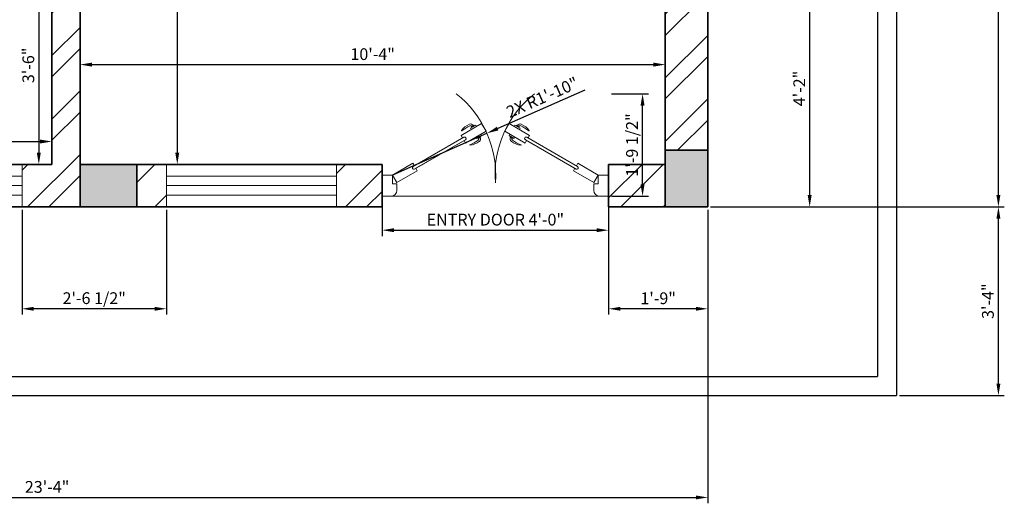
# Model space of a CAD drawing. Units: inches. Extents: x -138 to 270, y 8284 to 8764.
# Tile 5 of 10: x 61 to 270, y 8284 to 8387. Entities that reach past the tile are written whole.
import ezdxf

# ---------------------------------------------------------------- set-up
doc = ezdxf.new("R2010")
doc.units = ezdxf.units.IN
for name, color, linetype, lineweight in [('A-ANNO-DIMS', 2, 'Continuous', 18), ('C-PROP', 7, 'Continuous', 25), ('DOOR', 32, 'Continuous', 15), ('WALL', 8, 'Continuous', 35), ('WINDOW', 151, 'Continuous', 15)]:
    doc.layers.add(name, color=color, linetype=linetype, lineweight=lineweight)
doc.layers.add('A-COLS', color=252, linetype='Continuous', lineweight=35, true_color=0x939598)
doc.layers.add('A-WALL-PATT', color=32, linetype='Continuous', lineweight=9, true_color=0xbc761a)
doc.styles.get("Standard").update_dxf_attribs({"font": 'arial.ttf'})
doc.dimstyles.new('ISO-25', dxfattribs={"dimtxt": 2.5, "dimasz": 2.5, "dimexe": 1.25, "dimexo": 0.625, "dimtad": 1, "dimdec": 0, "dimlunit": 3, "dimtxsty": 'Standard', "dimcen": 2.5, "dimadec": 0, "dimazin": 0, "dimtfac": 1, "dimtdec": 0, "dimtmove": 0, "dimatfit": 3, "dimfxl": 1, "dimarcsym": 0})

# ---------------------------------------------------------------- blocks, each defined once
blk = doc.blocks.new('A$C441550E7')
at = {"layer": 'DOOR'}
for p, q in [((16.75, 12.91), (21.08, 15.41)), ((18.76, 14.43), (19.84, 15.05)), ((18.93, 14.75), (19.47, 15.06)), ((18.93, 14.75), (19.03, 14.58)), ((18.93, 14.75), (18.93, 14.75)), ((19.2, 14.9), (19.2, 14.9)), ((19.47, 15.06), (19.57, 14.9)), ((19.84, 15.05), (20, 14.78)), ((22.02, 13.78), (21.08, 15.41)), ((25.98, 13.78), (26.92, 15.41)), ((31.25, 12.91), (26.92, 15.41)), ((28.16, 15.05), (28, 14.78)), ((29.24, 14.43), (28.16, 15.05)), ((28.53, 15.06), (28.43, 14.9)), ((29.07, 14.75), (28.53, 15.06)), ((28.8, 14.9), (28.8, 14.9)), ((29.07, 14.75), (28.97, 14.58)), ((29.07, 14.75), (29.07, 14.75)), ((6.56, 6.3), (17.33, 12.52)), ((17.06, 12.36), (16.75, 12.91)), ((17.69, 11.28), (22.02, 13.78)), ((18.76, 14.43), (18.91, 14.16)), ((20.01, 12.26), (19.85, 12.53)), ((20.01, 12.26), (21.09, 12.89)), ((20.37, 12.26), (20.91, 12.57)), ((20.91, 12.57), (20.82, 12.73)), ((21.09, 12.89), (20.93, 13.16)), ((30.31, 11.28), (25.98, 13.78)), ((26.91, 12.89), (27.07, 13.16)), ((27.99, 12.26), (26.91, 12.89)), ((27.09, 12.57), (27.18, 12.73)), ((27.63, 12.26), (27.09, 12.57)), ((27.99, 12.26), (28.15, 12.53)), ((29.24, 14.43), (29.09, 14.16)), ((41.44, 6.3), (30.67, 12.52)), ((30.94, 12.36), (31.25, 12.91)), ((17.64, 11.98), (6.87, 5.76)), ((7.14, 5.92), (17.37, 11.82)), ((17.69, 11.28), (17.37, 11.82)), ((17.76, 12.41), (17.76, 12.41)), ((20.37, 12.26), (20.28, 12.42)), ((20.37, 12.26), (20.37, 12.26)), ((20.64, 12.41), (20.64, 12.41)), ((27.36, 12.41), (27.36, 12.41)), ((27.63, 12.26), (27.72, 12.42)), ((27.63, 12.26), (27.63, 12.26)), ((30.24, 12.41), (30.24, 12.41)), ((30.31, 11.28), (30.63, 11.82)), ((30.36, 11.98), (41.13, 5.76)), ((40.86, 5.92), (30.63, 11.82)), ((6.52, 7), (2.19, 4.5)), ((6.83, 6.46), (6.52, 7)), ((41.17, 6.46), (41.48, 7)), ((41.48, 7), (45.81, 4.5)), ((0, 0), (0, 4.5)), ((0, 4.5), (2.19, 4.5)), ((2.19, 2.62), (2.19, 4.5)), ((3.12, 2.88), (2.19, 4.5)), ((7.46, 5.38), (3.12, 2.88)), ((6.45, 5.88), (6.45, 5.88)), ((7.46, 5.38), (7.14, 5.92)), ((40.54, 5.38), (40.86, 5.92)), ((40.54, 5.38), (44.87, 2.88)), ((41.55, 5.88), (41.55, 5.88)), ((44.87, 2.88), (45.81, 4.5)), ((48, 4.5), (45.81, 4.5)), ((45.81, 2.62), (45.81, 4.5)), ((48, 0), (48, 4.5)), ((2.19, 2.62), (3.12, 2.62)), ((3.12, 1.25), (3.12, 2.62)), ((44.87, 1.25), (44.87, 2.62)), ((45.81, 2.62), (44.87, 2.62)), ((0, 0), (1.87, 0)), ((0, 0), (48, 0)), ((48, 0), (46.12, 0))]:
    blk.add_line(p, q, dxfattribs=at)
at = {"layer": 'DOOR', "ltscale": 0.1}
for centre, start, end in [((2.3, 4.56), 355.5279, 52.0858), ((45.7, 4.56), 127.9142, 184.4721)]:
    blk.add_arc(centre, 21.77, start, end, dxfattribs=at)
at = {"layer": 'DOOR'}
for centre, radius, start, end in [((19.83, 11.88), 3.63, 111.4546, 145.7774), ((22.15, 7.07), 8.61, 114.2033, 127.709), ((18.77, 14.74), 0.592, 22.7059, 117.5689), ((18.78, 14.66), 0.312, 30, 120), ((29.23, 14.74), 0.592, 62.4311, 157.2941), ((29.22, 14.66), 0.312, 60, 150), ((25.85, 7.07), 8.61, 52.291, 65.7967), ((28.17, 11.88), 3.63, 34.2226, 68.5454), ((16.85, 13.9), 0.0372, 138.2373, 332.5518), ((17.49, 12.25), 0.312, 30, 120), ((30.51, 12.25), 0.312, 60, 150), ((31.15, 13.9), 0.0372, 207.4482, 41.7627), ((17.49, 12.25), 0.312, 300, 30), ((18.6, 10.88), 0.0372, 87.4482, 281.7627), ((15.33, 18.88), 8.61, 292.291, 305.7967), ((18.34, 14.46), 3.63, 274.2226, 308.5454), ((20.22, 12.17), 0.312, 300, 30), ((20.29, 12.12), 0.592, 302.4311, 37.2941), ((27.71, 12.12), 0.592, 142.7059, 237.5689), ((29.66, 14.46), 3.63, 231.4546, 265.7774), ((27.78, 12.17), 0.312, 150, 240), ((32.67, 18.88), 8.61, 234.2033, 247.709), ((29.4, 10.88), 0.0372, 258.2373, 92.5518), ((30.51, 12.25), 0.312, 150, 240), ((6.72, 6.03), 0.312, 120, 210), ((41.28, 6.03), 0.312, 330, 60), ((6.72, 6.03), 0.312, 210, 300), ((41.28, 6.03), 0.312, 240, 330), ((1.87, 1.25), 1.25, 270, 0), ((46.12, 1.25), 1.25, 180, 270)]:
    blk.add_arc(centre, radius, start, end, dxfattribs=at)
blk = doc.blocks.new('*D22')
at = {"layer": 'A-ANNO-DIMS', "color": 0, "lineweight": -2, "transparency": 16777216}
for p, q in [((94.04, 8484.24), (93.42, 8484.24)), ((94.67, 8481.74), (94.67, 8358.74)), ((94.04, 8356.24), (93.42, 8356.24))]:
    blk.add_line(p, q, dxfattribs=at)
at = {"layer": 'A-ANNO-DIMS', "color": 0, "transparency": 16777216}
for points in [[(94.25, 8481.74), (95.09, 8481.74), (94.67, 8484.24)], [(94.25, 8358.74), (95.09, 8358.74), (94.67, 8356.24)]]:
    blk.add_solid(points, dxfattribs=at)
at = {"layer": 'Defpoints', "color": 0, "transparency": 16777216}
for p in [(94.67, 8484.24), (94.67, 8356.24), (94.67, 8356.24)]:
    blk.add_point(p, dxfattribs=at)
at = {"layer": 'A-ANNO-DIMS', "color": 0, "transparency": 16777216, "insert": (92.77, 8420.24), "char_height": 2.5, "attachment_point": 5, "rotation": 90}
blk.add_mtext('10\'-8"', dxfattribs=at)
blk = doc.blocks.new('*D23')
at = {"layer": 'A-ANNO-DIMS', "color": 0, "lineweight": -2, "transparency": 16777216}
for p, q in [((74.08, 8376.44), (74.08, 8378.65)), ((198.08, 8376.44), (198.08, 8378.65)), ((76.58, 8377.4), (195.58, 8377.4))]:
    blk.add_line(p, q, dxfattribs=at)
at = {"layer": 'A-ANNO-DIMS', "color": 0, "transparency": 16777216}
for points in [[(76.58, 8377.82), (76.58, 8376.98), (74.08, 8377.4)], [(195.58, 8377.82), (195.58, 8376.98), (198.08, 8377.4)]]:
    blk.add_solid(points, dxfattribs=at)
at = {"layer": 'Defpoints', "color": 0, "transparency": 16777216}
for p in [(74.08, 8375.82), (198.08, 8377.4), (198.08, 8375.82)]:
    blk.add_point(p, dxfattribs=at)
at = {"layer": 'A-ANNO-DIMS', "color": 0, "transparency": 16777216, "insert": (136.08, 8379.3), "char_height": 2.5, "attachment_point": 5}
blk.add_mtext('10\'-4"', dxfattribs=at)
blk = doc.blocks.new('*D24')
at = {"layer": 'A-ANNO-DIMS', "color": 0, "lineweight": -2, "transparency": 16777216}
for p, q in [((32.08, 8356.87), (32.08, 8362.34)), ((68.08, 8356.87), (68.08, 8362.34)), ((34.58, 8361.09), (65.58, 8361.09))]:
    blk.add_line(p, q, dxfattribs=at)
at = {"layer": 'A-ANNO-DIMS', "color": 0, "transparency": 16777216}
for points in [[(34.58, 8361.51), (34.58, 8360.67), (32.08, 8361.09)], [(65.58, 8361.51), (65.58, 8360.67), (68.08, 8361.09)]]:
    blk.add_solid(points, dxfattribs=at)
at = {"layer": 'Defpoints', "color": 0, "transparency": 16777216}
for p in [(68.08, 8361.09), (32.08, 8356.24), (68.08, 8356.24)]:
    blk.add_point(p, dxfattribs=at)
at = {"layer": 'A-ANNO-DIMS', "color": 0, "transparency": 16777216, "insert": (50.08, 8362.99), "char_height": 2.5, "attachment_point": 5}
blk.add_mtext("3'", dxfattribs=at)
blk = doc.blocks.new('*D25')
at = {"layer": 'A-ANNO-DIMS', "color": 0, "lineweight": -2, "transparency": 16777216}
for p, q in [((67.45, 8398.24), (64.08, 8398.24)), ((65.33, 8395.74), (65.33, 8358.74)), ((67.45, 8356.24), (64.08, 8356.24))]:
    blk.add_line(p, q, dxfattribs=at)
at = {"layer": 'A-ANNO-DIMS', "color": 0, "transparency": 16777216}
for points in [[(64.91, 8395.74), (65.75, 8395.74), (65.33, 8398.24)], [(64.91, 8358.74), (65.75, 8358.74), (65.33, 8356.24)]]:
    blk.add_solid(points, dxfattribs=at)
at = {"layer": 'Defpoints', "color": 0, "transparency": 16777216}
for p in [(68.08, 8398.24), (65.33, 8356.24), (68.08, 8356.24)]:
    blk.add_point(p, dxfattribs=at)
at = {"layer": 'A-ANNO-DIMS', "color": 0, "transparency": 16777216, "insert": (63.43, 8377.24), "char_height": 2.5, "attachment_point": 5, "rotation": 90}
blk.add_mtext('3\'-6"', dxfattribs=at)
blk = doc.blocks.new('WINDOW-36IN')
for p, q in [((0, 6.5), (36, 6.5)), ((0, 4.5), (36, 4.5)), ((0, 2.5), (36, 2.5))]:
    blk.add_line(p, q)
blk.add_lwpolyline([(0, 0), (36, 0), (36, 9), (0, 9)], close=True)
blk = doc.blocks.new('WINDOW-24IN')
for p, q in [((0, 6.5), (24, 6.5)), ((0, 4.5), (24, 4.5)), ((0, 2.5), (24, 2.5))]:
    blk.add_line(p, q)
blk.add_lwpolyline([(0, 0), (24, 0), (24, 9), (0, 9)], close=True)
blk = doc.blocks.new('COLUMN-9X12IN')
h = blk.add_hatch(color=256)
h.dxf.hatch_style = 1
h.paths.add_polyline_path([(9, 12), (0, 12), (0, 0), (9, 0)])
blk.add_lwpolyline([(0, 0), (9, 0), (9, 12), (0, 12)], close=True)
blk = doc.blocks.new('*D49')
at = {"layer": 'A-ANNO-DIMS', "color": 0, "lineweight": -2, "transparency": 16777216}
for p, q in [((138.08, 8348.87), (138.08, 8341.04)), ((186.08, 8348.87), (186.08, 8341.04)), ((140.58, 8342.29), (183.58, 8342.29))]:
    blk.add_line(p, q, dxfattribs=at)
at = {"layer": 'A-ANNO-DIMS', "color": 0, "transparency": 16777216}
for points in [[(140.58, 8342.71), (140.58, 8341.88), (138.08, 8342.29)], [(183.58, 8342.71), (183.58, 8341.88), (186.08, 8342.29)]]:
    blk.add_solid(points, dxfattribs=at)
at = {"layer": 'Defpoints', "color": 0, "transparency": 16777216}
for p in [(138.08, 8349.49), (186.08, 8349.49), (186.08, 8342.29)]:
    blk.add_point(p, dxfattribs=at)
at = {"layer": 'A-ANNO-DIMS', "color": 0, "transparency": 16777216, "insert": (162.08, 8344.21), "char_height": 2.5, "attachment_point": 5}
blk.add_mtext('ENTRY DOOR 4\'-0"', dxfattribs=at)
blk = doc.blocks.new('*D50')
at = {"layer": 'A-ANNO-DIMS', "color": 0, "lineweight": -2, "transparency": 16777216}
for p, q in [((186.7, 8371.22), (194.53, 8371.22)), ((193.28, 8351.99), (193.28, 8368.72)), ((186.7, 8349.49), (194.53, 8349.49))]:
    blk.add_line(p, q, dxfattribs=at)
at = {"layer": 'A-ANNO-DIMS', "color": 0, "transparency": 16777216}
for points in [[(192.86, 8368.72), (193.69, 8368.72), (193.28, 8371.22)], [(192.86, 8351.99), (193.69, 8351.99), (193.28, 8349.49)]]:
    blk.add_solid(points, dxfattribs=at)
at = {"layer": 'Defpoints', "color": 0, "transparency": 16777216}
for p in [(186.08, 8371.22), (193.28, 8371.22), (186.08, 8349.49)]:
    blk.add_point(p, dxfattribs=at)
at = {"layer": 'A-ANNO-DIMS', "color": 0, "transparency": 16777216, "insert": (191.36, 8360.36), "char_height": 2.5, "attachment_point": 5, "rotation": 90}
blk.add_mtext('1\'-9 1/2"', dxfattribs=at)
blk = doc.blocks.new('*D53')
at = {"layer": 'A-ANNO-DIMS', "color": 0, "lineweight": -2, "transparency": 16777216}
for p, q in [((-72.92, 8346.62), (-72.92, 8284.38)), ((207.08, 8346.62), (207.08, 8284.38)), ((-70.42, 8285.63), (204.58, 8285.63))]:
    blk.add_line(p, q, dxfattribs=at)
at = {"layer": 'A-ANNO-DIMS', "color": 0, "transparency": 16777216}
for points in [[(-70.42, 8286.04), (-70.42, 8285.21), (-72.92, 8285.63)], [(204.58, 8286.04), (204.58, 8285.21), (207.08, 8285.63)]]:
    blk.add_solid(points, dxfattribs=at)
at = {"layer": 'Defpoints', "color": 0, "transparency": 16777216}
for p in [(-72.92, 8347.24), (207.08, 8347.24), (207.08, 8285.63)]:
    blk.add_point(p, dxfattribs=at)
at = {"layer": 'A-ANNO-DIMS', "color": 0, "transparency": 16777216, "insert": (67.08, 8287.53), "char_height": 2.5, "attachment_point": 5}
blk.add_mtext('23\'-4"', dxfattribs=at)
blk = doc.blocks.new('*D54')
at = {"layer": 'A-ANNO-DIMS', "color": 0, "lineweight": -2, "transparency": 16777216}
for p, q in [((207.7, 8699.24), (269.94, 8699.24)), ((268.69, 8349.74), (268.69, 8696.74)), ((207.7, 8347.24), (269.94, 8347.24))]:
    blk.add_line(p, q, dxfattribs=at)
at = {"layer": 'A-ANNO-DIMS', "color": 0, "transparency": 16777216}
for points in [[(268.27, 8696.74), (269.11, 8696.74), (268.69, 8699.24)], [(268.27, 8349.74), (269.11, 8349.74), (268.69, 8347.24)]]:
    blk.add_solid(points, dxfattribs=at)
at = {"layer": 'Defpoints', "color": 0, "transparency": 16777216}
for p in [(207.08, 8699.24), (268.69, 8699.24), (207.08, 8347.24)]:
    blk.add_point(p, dxfattribs=at)
at = {"layer": 'A-ANNO-DIMS', "color": 0, "transparency": 16777216, "insert": (266.79, 8523.24), "char_height": 2.5, "attachment_point": 5, "rotation": 90}
blk.add_mtext('29\'-4"', dxfattribs=at)
blk = doc.blocks.new('*D56')
at = {"layer": 'A-ANNO-DIMS', "color": 0, "lineweight": -2, "transparency": 16777216}
for p, q in [((207.7, 8347.24), (269.94, 8347.24)), ((268.69, 8309.74), (268.69, 8344.74)), ((247.7, 8307.24), (269.94, 8307.24))]:
    blk.add_line(p, q, dxfattribs=at)
at = {"layer": 'A-ANNO-DIMS', "color": 0, "transparency": 16777216}
for points in [[(268.27, 8344.74), (269.11, 8344.74), (268.69, 8347.24)], [(268.27, 8309.74), (269.11, 8309.74), (268.69, 8307.24)]]:
    blk.add_solid(points, dxfattribs=at)
at = {"layer": 'Defpoints', "color": 0, "transparency": 16777216}
for p in [(207.08, 8347.24), (268.69, 8347.24), (247.08, 8307.24)]:
    blk.add_point(p, dxfattribs=at)
at = {"layer": 'A-ANNO-DIMS', "color": 0, "transparency": 16777216, "insert": (266.79, 8327.24), "char_height": 2.5, "attachment_point": 5, "rotation": 90}
blk.add_mtext('3\'-4"', dxfattribs=at)
blk = doc.blocks.new('*D57')
at = {"layer": 'A-ANNO-DIMS', "color": 0, "lineweight": -2, "transparency": 16777216}
for p, q in [((186.08, 8346.62), (186.08, 8324.38)), ((207.08, 8346.62), (207.08, 8324.38)), ((204.58, 8325.63), (188.58, 8325.63))]:
    blk.add_line(p, q, dxfattribs=at)
at = {"layer": 'A-ANNO-DIMS', "color": 0, "transparency": 16777216}
for points in [[(188.58, 8326.04), (188.58, 8325.21), (186.08, 8325.63)], [(204.58, 8326.04), (204.58, 8325.21), (207.08, 8325.63)]]:
    blk.add_solid(points, dxfattribs=at)
at = {"layer": 'Defpoints', "color": 0, "transparency": 16777216}
for p in [(186.08, 8347.24), (207.08, 8347.24), (186.08, 8325.63)]:
    blk.add_point(p, dxfattribs=at)
at = {"layer": 'A-ANNO-DIMS', "color": 0, "transparency": 16777216, "insert": (196.58, 8327.53), "char_height": 2.5, "attachment_point": 5}
blk.add_mtext('1\'-9"', dxfattribs=at)
blk = doc.blocks.new('*D60')
at = {"layer": 'A-ANNO-DIMS', "color": 0, "lineweight": -2, "transparency": 16777216}
for p, q in [((61.77, 8346.62), (61.77, 8324.38)), ((92.38, 8346.62), (92.38, 8324.38)), ((89.88, 8325.63), (64.27, 8325.63))]:
    blk.add_line(p, q, dxfattribs=at)
at = {"layer": 'A-ANNO-DIMS', "color": 0, "transparency": 16777216}
for points in [[(64.27, 8326.04), (64.27, 8325.21), (61.77, 8325.63)], [(89.88, 8326.04), (89.88, 8325.21), (92.38, 8325.63)]]:
    blk.add_solid(points, dxfattribs=at)
at = {"layer": 'Defpoints', "color": 0, "transparency": 16777216}
for p in [(61.77, 8347.24), (92.38, 8347.24), (61.77, 8325.63)]:
    blk.add_point(p, dxfattribs=at)
at = {"layer": 'A-ANNO-DIMS', "color": 0, "transparency": 16777216, "insert": (77.07, 8327.55), "char_height": 2.5, "attachment_point": 5}
blk.add_mtext('2\'-6 1/2"', dxfattribs=at)
blk = doc.blocks.new('*D67')
at = {"layer": 'A-ANNO-DIMS', "color": 0, "lineweight": -2, "transparency": 16777216}
for p, q in [((207.7, 8397.43), (229.94, 8397.43)), ((228.69, 8394.93), (228.69, 8349.74)), ((207.7, 8347.24), (229.94, 8347.24))]:
    blk.add_line(p, q, dxfattribs=at)
at = {"layer": 'A-ANNO-DIMS', "color": 0, "transparency": 16777216}
for points in [[(228.27, 8394.93), (229.11, 8394.93), (228.69, 8397.43)], [(228.27, 8349.74), (229.11, 8349.74), (228.69, 8347.24)]]:
    blk.add_solid(points, dxfattribs=at)
at = {"layer": 'Defpoints', "color": 0, "transparency": 16777216}
for p in [(207.08, 8397.43), (207.08, 8347.24), (228.69, 8347.24)]:
    blk.add_point(p, dxfattribs=at)
at = {"layer": 'A-ANNO-DIMS', "color": 0, "transparency": 16777216, "insert": (226.81, 8372.34), "char_height": 2.5, "attachment_point": 5, "rotation": 90}
blk.add_mtext('4\'-2"', dxfattribs=at)
blk = doc.blocks.new('*D78')
at = {"layer": 'A-ANNO-DIMS', "color": 0, "lineweight": -2, "transparency": 16777216}
for p, q in [((181.01, 8371.98), (162.58, 8363.85)), ((140.38, 8354.05), (160.29, 8362.84))]:
    blk.add_line(p, q, dxfattribs=at)
at = {"layer": 'A-ANNO-DIMS', "color": 0, "transparency": 16777216}
blk.add_solid([(162.41, 8364.23), (162.75, 8363.46), (160.29, 8362.84)], dxfattribs=at)
at = {"layer": 'Defpoints', "color": 0, "transparency": 16777216}
for p in [(160.29, 8362.84), (140.38, 8354.05)]:
    blk.add_point(p, dxfattribs=at)
at = {"layer": 'A-ANNO-DIMS', "color": 0, "transparency": 16777216, "insert": (172.17, 8370.16), "char_height": 2.5, "attachment_point": 5, "rotation": 23.8064}
blk.add_mtext('2X R1\'-10"', dxfattribs=at)

msp = doc.modelspace()

# ---------------------------------------------------------------- hatches: boundary and pattern name
at = {"layer": 'A-WALL-PATT'}
h = msp.add_hatch(dxfattribs=at)
h.set_pattern_fill('ANSI32', color=256)
h.paths.add_polyline_path([(115.81, 8699.24), (65.22, 8699.24), (65.22, 8690.24), (68.08, 8690.24), (68.08, 8686.36), (69.02, 8686.36), (69.02, 8686.36), (73.52, 8686.36), (74.08, 8686.36), (74.08, 8690.24), (115.81, 8690.24)])
h.paths.add_polyline_path([(169.81, 8699.24), (139.81, 8699.24), (139.81, 8690.24), (169.81, 8690.24)])
h.paths.add_polyline_path([(198.08, 8699.24), (193.81, 8699.24), (193.81, 8690.24), (198.08, 8690.24)])
h.paths.add_polyline_path([(207.08, 8648.24), (204.23, 8648.24), (204.23, 8648.24), (199.73, 8648.24), (198.08, 8648.24), (198.08, 8642.24), (150.08, 8642.24), (150.08, 8690.24), (144.08, 8690.24), (144.08, 8642.24), (74.08, 8642.24), (74.08, 8653.36), (68.08, 8653.36), (68.08, 8526.24), (68.83, 8526.24), (74.08, 8526.24), (74.08, 8630.24), (74.08, 8636.24), (98.08, 8636.24), (150.08, 8636.24), (198.08, 8636.24), (198.08, 8630.24), (198.08, 8532.24), (207.08, 8532.24)])
h.paths.add_polyline_path([(207.08, 8484.24), (198.08, 8484.24), (198.08, 8433.43), (207.08, 8433.43)])
h.paths.add_polyline_path([(198.08, 8490.24), (80.08, 8490.24), (80.08, 8484.24), (198.08, 8484.24)])
h.paths.add_polyline_path([(207.08, 8397.43), (198.08, 8397.43), (198.08, 8359.27), (207.08, 8359.27)])
h.paths.add_polyline_path([(198.08, 8356.24), (186.08, 8356.24), (186.08, 8347.24), (198.08, 8347.24)])
h.paths.add_polyline_path([(138.08, 8356.24), (128.38, 8356.24), (128.38, 8347.24), (138.08, 8347.24)])
h.paths.add_polyline_path([(92.38, 8356.24), (86.08, 8356.24), (86.08, 8347.24), (92.38, 8347.24)])
h = msp.add_hatch(dxfattribs=at)
h.set_pattern_fill('ANSI32', color=256)
h.paths.add_polyline_path([(-23.4, 8356.24), (-63.92, 8356.24), (-63.92, 8347.24), (-23.4, 8347.24)])
h.paths.add_polyline_path([(-63.92, 8469.84), (-72.92, 8469.84), (-72.92, 8359.24), (-63.92, 8359.24)])
h.paths.add_polyline_path([(-63.92, 8510.27), (-72.92, 8510.27), (-72.92, 8505.84), (-63.92, 8505.84)])
h.paths.add_polyline_path([(-63.92, 8527.36), (-72.92, 8527.36), (-72.92, 8522.27), (-63.92, 8522.27)])
h.paths.add_polyline_path([(26.08, 8522.24), (24.78, 8522.24), (24.78, 8522.24), (20.08, 8522.24), (20.08, 8516.24), (-63.92, 8516.24), (-63.92, 8510.24), (26.08, 8510.24)])
h.paths.add_polyline_path([(34.02, 8398.24), (34.02, 8404.24), (26.08, 8404.24), (26.08, 8356.24), (12.6, 8356.24), (12.6, 8347.24), (37.77, 8347.24), (37.77, 8356.24), (32.08, 8356.24), (32.08, 8398.24)])
h.paths.add_polyline_path([(67.02, 8404.24), (67.02, 8398.24), (68.08, 8398.24), (68.08, 8356.24), (61.77, 8356.24), (61.77, 8347.24), (74.08, 8347.24), (74.08, 8356.24), (74.08, 8356.24), (74.08, 8449.75), (68.08, 8449.75), (68.08, 8404.24)])

# ---------------------------------------------------------------- linework, layer by layer
at = {"layer": 'C-PROP'}
for p, q in [((247.08, 8739.24), (247.08, 8307.24)), ((243.08, 8735.24), (243.08, 8311.24)), ((-108.92, 8311.24), (243.08, 8311.24)), ((198.08, 8311.24), (243.08, 8311.24)), ((-112.92, 8307.24), (247.08, 8307.24))]:
    msp.add_line(p, q, dxfattribs=at)
at = {"layer": 'WALL'}
for p, q in [((207.08, 8648.24), (207.08, 8347.24)), ((198.08, 8484.24), (198.08, 8356.24)), ((74.08, 8449.75), (74.08, 8356.24)), ((68.08, 8398.24), (68.08, 8356.24)), ((32.08, 8356.24), (68.08, 8356.24)), ((74.08, 8356.24), (138.08, 8356.24)), ((138.08, 8356.24), (138.08, 8347.24)), ((186.08, 8347.24), (186.08, 8356.24)), ((186.08, 8356.24), (198.08, 8356.24)), ((42.08, 8347.24), (138.08, 8347.24)), ((186.08, 8347.24), (207.08, 8347.24))]:
    msp.add_line(p, q, dxfattribs=at)

# ---------------------------------------------------------------- block references
at = {"layer": 'A-COLS'}
msp.add_blockref('COLUMN-9X12IN', (198.08, 8347.27), dxfattribs=at)
at = {"layer": 'A-COLS', "rotation": 90.00000000000006}
msp.add_blockref('COLUMN-9X12IN', (86.08, 8347.24), dxfattribs=at)
at = {"layer": 'DOOR'}
msp.add_blockref('A$C441550E7', (138.08, 8349.49), dxfattribs=at)
at = {"layer": 'WINDOW'}
for name, p in [('WINDOW-24IN', (37.77, 8347.24)), ('WINDOW-36IN', (92.38, 8347.24))]:
    msp.add_blockref(name, p, dxfattribs=at)

# ---------------------------------------------------------------- dimensions: what is measured, and where the dimension line sits
at = {"layer": 'A-ANNO-DIMS'}
for base, p1, p2, angle, picture, middle in [((268.69, 8699.24), (207.08, 8347.24), (207.08, 8699.24), 90, '*D54', (266.79, 8523.24)), ((228.69, 8347.24), (207.08, 8397.43), (207.08, 8347.24), 270, '*D67', (226.81, 8372.34)), ((193.28, 8371.22), (186.08, 8349.49), (186.08, 8371.22), 90, '*D50', (191.36, 8360.36)), ((61.77, 8325.63), (92.38, 8347.24), (61.77, 8347.24), 180, '*D60', (77.07, 8327.55)), ((186.08, 8325.63), (207.08, 8347.24), (186.08, 8347.24), 180, '*D57', (196.58, 8327.53)), ((268.69, 8347.24), (247.08, 8307.24), (207.08, 8347.24), 90, '*D56', (266.79, 8327.24))]:
    dim = msp.add_linear_dim(base=base, p1=p1, p2=p2, angle=angle, dimstyle='ISO-25', override={"dimdec": 1, "dimlfac": 1, "dimrnd": 0, "dimzin": 1, "dimdsep": 46, "dimlunit": 4, "dimfrac": 2}, dxfattribs=at)
    dim.commit()
    dim.dimension.update_dxf_attribs({"geometry": picture, "text_midpoint": middle})
for p1, p2, distance, picture, middle in [((94.67, 8484.24), (94.67, 8356.24), 0, '*D22', (92.77, 8420.24)), ((68.08, 8398.24), (68.08, 8356.24), -2.75, '*D25', (63.43, 8377.24)), ((74.08, 8375.82), (198.08, 8375.82), 1.58, '*D23', (136.08, 8379.3)), ((32.08, 8356.24), (68.08, 8356.24), 4.85, '*D24', (50.08, 8362.99))]:
    dim = msp.add_aligned_dim(p1=p1, p2=p2, distance=distance, dimstyle='ISO-25', override={"dimclrd": 0, "dimclre": 0, "dimclrt": 0}, dxfattribs=at)
    dim.commit()
    dim.dimension.update_dxf_attribs({"geometry": picture, "text_midpoint": middle})
dim = msp.add_radius_dim(center=(140.38, 8354.05), mpoint=(160.29, 8362.84), text='2X <>', dimstyle='ISO-25', override={"dimdec": 1, "dimlfac": 1, "dimrnd": 0, "dimzin": 1, "dimdsep": 46, "dimlunit": 4, "dimfrac": 2}, dxfattribs=at)
dim.commit()
dim.dimension.update_dxf_attribs({"geometry": '*D78', "text_midpoint": (172.17, 8370.16)})
dim = msp.add_linear_dim(base=(186.08, 8342.29), p1=(138.08, 8349.49), p2=(186.08, 8349.49), text='ENTRY DOOR <>', dimstyle='ISO-25', override={"dimdec": 1, "dimlfac": 1, "dimrnd": 0, "dimzin": 1, "dimdsep": 46, "dimlunit": 4, "dimfrac": 2}, dxfattribs=at)
dim.commit()
dim.dimension.update_dxf_attribs({"geometry": '*D49', "text_midpoint": (162.08, 8344.21)})
dim = msp.add_linear_dim(base=(207.08, 8285.63), p1=(-72.92, 8347.24), p2=(207.08, 8347.24), dimstyle='ISO-25', override={"dimdec": 1, "dimlfac": 1, "dimrnd": 0, "dimzin": 1, "dimdsep": 46, "dimlunit": 4, "dimfrac": 2}, dxfattribs=at)
dim.commit()
dim.dimension.update_dxf_attribs({"geometry": '*D53', "text_midpoint": (67.08, 8287.53)})

doc.saveas('drawing.dxf')
